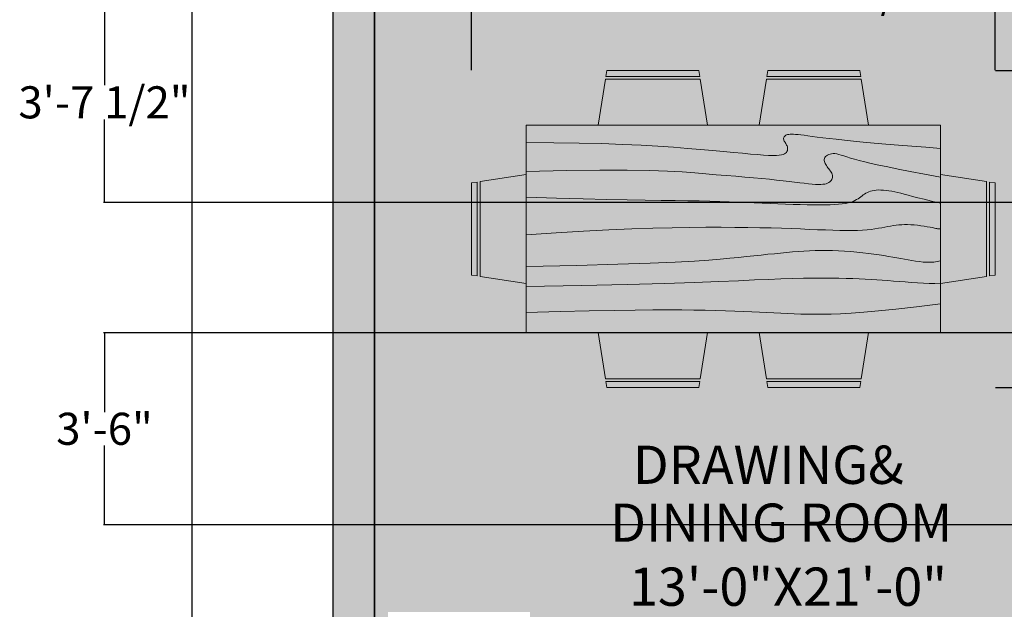
# Model space of a CAD drawing. Units: inches. Extents: x 1884 to 2398, y 474 to 1488.
# Tile 31 of 39: x 1884 to 2099, y 761 to 889. Entities that reach past the tile are written whole.
import ezdxf

# ---------------------------------------------------------------- set-up
doc = ezdxf.new("R2010")
doc.units = ezdxf.units.IN
doc.header["$MEASUREMENT"] = 0
doc.layers.get('0').update_dxf_attribs({"color": 250})
for name, color, linetype, lineweight in [('A-ANNO-DIMS', 2, 'Continuous', 18), ('A-AREA-IDEN', 7, 'Continuous', 18), ('A-FLOR-PATT', 254, 'Continuous', 13), ('A-FURN-PATT', 253, 'Continuous', 13), ('A-WALL-PATT', 250, 'Continuous', 13), ('C-PROP', 7, 'Continuous', 30), ('furniture', 8, 'Continuous', 18), ('walls', 7, 'Continuous', 35)]:
    doc.layers.add(name, color=color, linetype=linetype, lineweight=lineweight)
doc.styles.get("Standard").update_dxf_attribs({"font": 'arial.ttf'})
doc.dimstyles.get("Standard").update_dxf_attribs({"dimtxt": 7, "dimasz": 0.18, "dimexe": 0.18, "dimexo": 0.0625, "dimgap": 0.09, "dimtad": 0, "dimtih": 1, "dimtoh": 1, "dimzin": 0, "dimdsep": 46, "dimlunit": 3, "dimtxsty": 'Standard', "dimcen": 0.09, "dimadec": 0, "dimazin": 0, "dimtfac": 1, "dimtofl": 0, "dimtmove": 0, "dimatfit": 3, "dimfxl": 1, "dimtolj": 1, "dimtzin": 0, "dimarcsym": 0})

# ---------------------------------------------------------------- blocks, each defined once
blk = doc.blocks.new('*D2')
at = {"layer": 'A-ANNO-DIMS', "color": 0, "lineweight": -2, "transparency": 16777216}
for p, q in [((1920.51, 1406.88), (1921.96, 1406.88)), ((1921.78, 1406.7), (1921.78, 972.55)), ((1921.78, 531.06), (1921.78, 965.22)), ((1920.51, 530.88), (1921.96, 530.88))]:
    blk.add_line(p, q, dxfattribs=at)
at = {"layer": 'A-ANNO-DIMS', "color": 0, "lineweight": 100, "transparency": 16777216}
for points in [[(1921.75, 1406.7), (1921.81, 1406.7), (1921.78, 1406.88)], [(1921.75, 531.06), (1921.81, 531.06), (1921.78, 530.88)]]:
    blk.add_solid(points, dxfattribs=at)
at = {"layer": 'Defpoints', "color": 0, "lineweight": 100, "transparency": 16777216}
for p in [(1920.45, 1406.88), (1920.45, 530.88), (1921.78, 530.88)]:
    blk.add_point(p, dxfattribs=at)
at = {"layer": 'A-ANNO-DIMS', "color": 0, "transparency": 16777216, "insert": (1921.78, 968.88), "char_height": 7, "attachment_point": 5}
blk.add_mtext("\\A1;73'", dxfattribs=at)
blk = doc.blocks.new('Dining Set - 36 x 72 in.')
for p, q in [((-22, 27.5), (-22.1562, 26.50042)), ((-22, 27.5), (-6, 27.5)), ((-5.8437, 26.49966), (-6, 27.5)), ((6, 27.5), (5.8438, 26.50042)), ((6, 27.5), (22, 27.5)), ((22.1563, 26.49966), (22, 27.5)), ((-22.2343, 26.00059), (-23.4847, 17.99762)), ((-22.2304, 26), (-5.7608, 26)), ((-5.8416, 26.5), (-22.1534, 26.5)), ((-4.5152, 17.99762), (-5.7655, 25.99926)), ((5.7657, 26.00059), (4.5153, 17.99762)), ((5.7696, 26), (22.2392, 26)), ((22.1584, 26.5), (5.8466, 26.5)), ((23.4848, 17.99762), (22.2345, 25.99926)), ((36, 18), (-36, 18)), ((-36, 18), (-36, -18)), ((36, -18), (36, 18)), ((-44.0006, 8.23428), (-35.9976, 9.48474)), ((44.0006, 8.23428), (35.9976, 9.48474)), ((-45.5, 8), (-44.5004, 8.15617)), ((-45.5, 8), (-45.5, -8)), ((-44.5, -8.15843), (-44.5, 8.15338)), ((-44, 8.23041), (-44, -8.23915)), ((44, 8.23041), (44, -8.23915)), ((44.5, -8.15843), (44.5, 8.15338)), ((45.5, 8), (44.5005, 8.15617)), ((45.5, 8), (45.5, -8)), ((-44.4997, -8.15631), (-45.5, -8)), ((-35.9976, -9.48476), (-43.9993, -8.2345)), ((35.9976, -9.48476), (43.9993, -8.2345)), ((44.4997, -8.15631), (45.5, -8)), ((-36, -18), (36, -18)), ((-22.2343, -26.0006), (-23.4847, -17.99762)), ((-4.5152, -17.99762), (-5.7655, -25.99928)), ((5.7657, -26.0006), (4.5153, -17.99762)), ((23.4848, -17.99762), (22.2345, -25.99928)), ((-22.2304, -26), (-5.7608, -26)), ((-22, -27.5), (-22.1562, -26.50044)), ((-5.8416, -26.5), (-22.1534, -26.5)), ((-5.8437, -26.49967), (-6, -27.5)), ((5.7696, -26), (22.2392, -26)), ((6, -27.5), (5.8438, -26.50044)), ((22.1584, -26.5), (5.8466, -26.5)), ((22.1563, -26.49967), (22, -27.5)), ((-22, -27.5), (-6, -27.5)), ((6, -27.5), (22, -27.5))]:
    blk.add_line(p, q)
for points in [[(-36, 15), (-31.1772, 14.97754), (-26.8079, 14.91406), (-22.8538, 14.81543), (-19.276, 14.6875), (-16.0362, 14.53613), (-13.0957, 14.36718), (-10.4159, 14.18652), (-7.9583, 14), (-5.6904, 13.81315), (-3.6035, 13.63021), (-1.6954, 13.45508), (0.0365, 13.29166), (1.5945, 13.14388), (2.9811, 13.01562), (4.1988, 12.9108), (5.25, 12.83333), (6.1393, 12.78613), (6.8802, 12.76823), (7.4883, 12.77767), (7.9792, 12.8125), (8.3685, 12.87077), (8.6719, 12.95052), (8.9049, 13.0498), (9.0833, 13.16666), (9.2205, 13.29899), (9.3216, 13.44401), (9.3895, 13.59879), (9.4271, 13.76041), (9.4373, 13.92594), (9.4232, 14.09245), (9.3875, 14.257), (9.3333, 14.41666), (9.2638, 14.56917), (9.1836, 14.71484), (9.0975, 14.85465), (9.0104, 14.98958), (8.9272, 15.1206), (8.8529, 15.2487), (8.7922, 15.37483), (8.75, 15.5), (8.7305, 15.62467), (8.7344, 15.74739), (8.7617, 15.86621), (8.8125, 15.97916), (8.8867, 16.08431), (8.9844, 16.17968), (9.1055, 16.26334), (9.25, 16.33333), (9.4189, 16.38802), (9.6172, 16.42708), (9.8506, 16.45052), (10.125, 16.45833), (10.4463, 16.45052), (10.8203, 16.42708), (11.2529, 16.38802), (11.75, 16.33333), (12.3184, 16.26318), (12.9694, 16.17838), (13.7151, 16.07991), (14.5677, 15.96875), (15.5395, 15.84586), (16.6426, 15.71224), (17.8893, 15.56884), (19.2917, 15.41666), (20.859, 15.25667), (22.5879, 15.08984), (24.4721, 14.91715), (26.5052, 14.73958), (28.6809, 14.5581), (30.9929, 14.3737), (33.4347, 14.18733), (36, 14)], [(-36, 10), (-28.9766, 10.14274), (-23.1725, 10.20442), (-18.4241, 10.19775), (-14.5677, 10.13541), (-11.4399, 10.03011), (-8.877, 9.89453), (-6.7154, 9.74137), (-4.7917, 9.58333), (-2.9698, 9.43082), (-1.2246, 9.28515), (0.4415, 9.14534), (2.026, 9.01041), (3.5266, 8.87939), (4.9408, 8.7513), (6.266, 8.62516), (7.5, 8.5), (8.6411, 8.37549), (9.6914, 8.2539), (10.6538, 8.13818), (11.5312, 8.03125), (12.3267, 7.93603), (13.043, 7.85547), (13.6831, 7.79248), (14.25, 7.75), (14.7471, 7.7303), (15.1797, 7.73307), (15.5537, 7.75732), (15.875, 7.80208), (16.1494, 7.86637), (16.3828, 7.94922), (16.5811, 8.04964), (16.75, 8.16666), (16.8944, 8.29915), (17.0143, 8.44531), (17.1089, 8.60319), (17.1771, 8.77083), (17.218, 8.94629), (17.2305, 9.1276), (17.2137, 9.31282), (17.1667, 9.5), (17.0895, 9.6875), (16.987, 9.875), (16.8649, 10.0625), (16.7292, 10.25), (16.5856, 10.4375), (16.4401, 10.625), (16.2985, 10.8125), (16.1667, 11), (16.05, 11.18733), (15.9518, 11.3737), (15.8752, 11.5581), (15.8229, 11.73958), (15.798, 11.91715), (15.8034, 12.08984), (15.842, 12.25667), (15.9167, 12.41666), (16.0295, 12.56836), (16.1784, 12.70833), (16.3605, 12.83268), (16.5729, 12.9375), (16.8127, 13.01888), (17.0768, 13.07291), (17.3625, 13.0957), (17.6667, 13.08333), (17.9894, 13.03312), (18.3418, 12.94726), (18.7382, 12.82918), (19.1927, 12.68229), (19.7195, 12.51001), (20.3327, 12.31575), (21.0465, 12.10294), (21.875, 11.875), (22.8357, 11.63354), (23.959, 11.37304), (25.2786, 11.08618), (26.8282, 10.76562), (28.6414, 10.40405), (30.752, 9.99414), (33.1936, 9.52856), (36, 9)], [(-36, 5.5), (-30.7157, 5.3348), (-26.069, 5.20963), (-21.9946, 5.11767), (-18.4271, 5.05208), (-15.3009, 5.00602), (-12.5508, 4.97265), (-10.1112, 4.94515), (-7.9167, 4.91666), (-5.909, 4.88167), (-4.0586, 4.83984), (-2.3429, 4.79215), (-0.7396, 4.73958), (0.7739, 4.6831), (2.22, 4.6237), (3.6213, 4.56233), (5, 4.5), (6.373, 4.43782), (7.7344, 4.3776), (9.0723, 4.32129), (10.375, 4.27083), (11.6309, 4.22819), (12.8281, 4.19531), (13.9551, 4.17415), (15, 4.16666), (15.954, 4.17448), (16.819, 4.19791), (17.6001, 4.23698), (18.3021, 4.29166), (18.9299, 4.36198), (19.4883, 4.44791), (19.9823, 4.54948), (20.4167, 4.66666), (20.7969, 4.79899), (21.1302, 4.94401), (21.4245, 5.09879), (21.6875, 5.26041), (21.9271, 5.42594), (22.1511, 5.59245), (22.3672, 5.757), (22.5834, 5.91666), (22.8065, 6.06868), (23.0404, 6.21093), (23.2879, 6.34147), (23.5521, 6.45833), (23.8358, 6.55957), (24.142, 6.64323), (24.4735, 6.70735), (24.8334, 6.75), (25.2235, 6.76969), (25.642, 6.76692), (26.0858, 6.74267), (26.5521, 6.69791), (27.0379, 6.63362), (27.5404, 6.55078), (28.0565, 6.45036), (28.5834, 6.33333), (29.1242, 6.19987), (29.7071, 6.04687), (30.3661, 5.87044), (31.1354, 5.66666), (32.0493, 5.43164), (33.142, 5.16146), (34.4475, 4.85221), (36, 4.5)], [(-36, -1), (-30.7915, -0.6591), (-26.0195, -0.38216), (-21.6519, -0.16284), (-17.6563, 0.00521), (-14.0005, 0.12833), (-10.6523, 0.21289), (-7.5796, 0.26522), (-4.75, 0.29166), (-2.134, 0.29793), (0.2878, 0.28711), (2.5317, 0.26163), (4.6146, 0.22396), (6.5529, 0.17651), (8.3633, 0.12174), (10.0623, 0.06209), (11.6667, 0), (13.1899, -0.06201), (14.6341, -0.1211), (15.9982, -0.17432), (17.2813, -0.21875), (18.4823, -0.25147), (19.6003, -0.26953), (20.6343, -0.27002), (21.5834, -0.25), (22.4481, -0.20768), (23.2357, -0.14584), (23.9549, -0.06836), (24.6146, 0.02083), (25.2235, 0.11784), (25.7904, 0.21875), (26.3241, 0.31966), (26.8334, 0.41666), (27.3265, 0.50618), (27.8099, 0.58593), (28.2894, 0.65397), (28.7709, 0.70833), (29.2601, 0.74707), (29.763, 0.76823), (30.2855, 0.76985), (30.8334, 0.75), (31.4088, 0.70784), (31.9994, 0.64713), (32.589, 0.57275), (33.1615, 0.48958), (33.7008, 0.4025), (34.1908, 0.3164), (34.6153, 0.23616), (34.9584, 0.16666), (35.2099, 0.11165), (35.3848, 0.07031), (35.504, 0.04069), (35.5886, 0.02083), (35.6594, 0.00879), (35.7377, 0.0026), (35.8442, 0.00032), (36, 0)], [(-36, -6.5), (-27.1843, -6.31267), (-20.084, -6.1263), (-14.469, -5.9419), (-10.1094, -5.76042), (-6.7752, -5.58285), (-4.2363, -5.41016), (-2.2629, -5.24333), (-0.625, -5.08334), (0.8708, -4.93099), (2.2715, -4.78646), (3.5872, -4.64974), (4.8281, -4.52084), (6.0046, -4.39974), (7.127, -4.28646), (8.2053, -4.18099), (9.25, -4.08334), (10.2705, -3.99382), (11.2734, -3.91407), (12.2647, -3.84603), (13.25, -3.79167), (14.2354, -3.75293), (15.2266, -3.73177), (16.2295, -3.73015), (17.25, -3.75), (18.2912, -3.79248), (19.3451, -3.85547), (20.4009, -3.93604), (21.4479, -4.03125), (22.4754, -4.13819), (23.4727, -4.25391), (24.4289, -4.37549), (25.3334, -4.5), (26.1785, -4.62492), (26.9694, -4.74935), (27.7145, -4.87281), (28.4219, -4.99479), (29.1, -5.11483), (29.7572, -5.23242), (30.4016, -5.34709), (31.0417, -5.45834), (31.6837, -5.56437), (32.3262, -5.65821), (32.9658, -5.73153), (33.599, -5.77604), (34.2224, -5.78345), (34.8327, -5.74545), (35.4264, -5.65373), (36, -5.5)], [(-36, -10), (-26.4022, -9.81299), (-18.4675, -9.62891), (-11.9839, -9.45069), (-6.7396, -9.28125), (-2.5226, -9.12354), (0.8789, -8.98047), (3.6769, -8.85498), (6.0833, -8.75), (8.2767, -8.66765), (10.3021, -8.60677), (12.1712, -8.56543), (13.8958, -8.54167), (15.4876, -8.53353), (16.9583, -8.53907), (18.3197, -8.55632), (19.5834, -8.58334), (20.7616, -8.61841), (21.8685, -8.66081), (22.9188, -8.71004), (23.9271, -8.76563), (24.9081, -8.82707), (25.8763, -8.89388), (26.8465, -8.96558), (27.8334, -9.04167), (28.8474, -9.12118), (29.8828, -9.20117), (30.93, -9.27824), (31.9792, -9.34896), (33.0205, -9.40991), (34.0443, -9.45768), (35.0407, -9.48885), (36, -9.5)], [(-36, -14.5), (-30.0881, -14.33513), (-25.0332, -14.21224), (-20.7312, -14.12647), (-17.0781, -14.07292), (-13.97, -14.04671), (-11.3027, -14.04297), (-8.9724, -14.05681), (-6.875, -14.08334), (-4.9224, -14.11833), (-3.0905, -14.16016), (-1.3709, -14.20785), (0.2448, -14.26042), (1.7647, -14.3169), (3.1973, -14.3763), (4.5507, -14.43767), (5.8333, -14.5), (7.0554, -14.5621), (8.235, -14.62175), (9.3922, -14.67652), (10.5469, -14.72396), (11.7192, -14.76164), (12.929, -14.78711), (14.1965, -14.79794), (15.5417, -14.79167), (16.9933, -14.76424), (18.6152, -14.70508), (20.4804, -14.60197), (22.6615, -14.44271), (25.2312, -14.21509), (28.2624, -13.9069), (31.8277, -13.50594), (36, -13)]]:
    blk.add_lwpolyline(points)
blk = doc.blocks.new('dining area')
at = {"layer": 'furniture', "xscale": 0.6659924291999282, "yscale": 0.6659924291999282, "zscale": 0.6659924291999282, "rotation": 90}
blk.add_blockref('Dining Set - 36 x 72 in.', (-0.44, 20.51), dxfattribs=at)
blk = doc.blocks.new('*D35')
at = {"layer": 'A-ANNO-DIMS', "color": 0, "lineweight": -2, "transparency": 16777216}
for p, q in [((1982.72, 878.09), (1982.72, 895.35)), ((1982.9, 895.17), (1993.17, 895.17)), ((2096.86, 895.17), (2086.6, 895.17)), ((2097.04, 878.09), (2097.04, 895.35))]:
    blk.add_line(p, q, dxfattribs=at)
at = {"layer": 'A-ANNO-DIMS', "color": 0, "lineweight": 100, "transparency": 16777216}
for points in [[(1982.9, 895.2), (1982.9, 895.14), (1982.72, 895.17)], [(2096.86, 895.2), (2096.86, 895.14), (2097.04, 895.17)]]:
    blk.add_solid(points, dxfattribs=at)
at = {"layer": 'Defpoints', "color": 0, "lineweight": 100, "transparency": 16777216}
for p in [(2097.04, 895.17), (1982.72, 878.02), (2097.04, 878.02)]:
    blk.add_point(p, dxfattribs=at)
at = {"layer": 'A-ANNO-DIMS', "color": 0, "transparency": 16777216, "insert": (2039.88, 895.17), "char_height": 7, "attachment_point": 5}
blk.add_mtext('\\A1;DINING SET 9\'-6 1/2"', dxfattribs=at)
blk = doc.blocks.new('*D36')
at = {"layer": 'A-ANNO-DIMS', "color": 0, "lineweight": -2, "transparency": 16777216}
for p, q in [((2097.11, 878.02), (2114.37, 878.02)), ((2114.19, 877.84), (2114.19, 847.14)), ((2114.19, 809.11), (2114.19, 839.81)), ((2097.11, 808.93), (2114.37, 808.93))]:
    blk.add_line(p, q, dxfattribs=at)
at = {"layer": 'A-ANNO-DIMS', "color": 0, "lineweight": 100, "transparency": 16777216}
for points in [[(2114.16, 877.84), (2114.22, 877.84), (2114.19, 878.02)], [(2114.16, 809.11), (2114.22, 809.11), (2114.19, 808.93)]]:
    blk.add_solid(points, dxfattribs=at)
at = {"layer": 'Defpoints', "color": 0, "lineweight": 100, "transparency": 16777216}
for p in [(2097.04, 878.02), (2097.04, 808.93), (2114.19, 808.93)]:
    blk.add_point(p, dxfattribs=at)
at = {"layer": 'A-ANNO-DIMS', "color": 0, "transparency": 16777216, "insert": (2114.19, 843.48), "char_height": 7, "attachment_point": 5}
blk.add_mtext('\\A1;5\'-9"', dxfattribs=at)
blk = doc.blocks.new('*D51')
at = {"layer": 'A-ANNO-DIMS', "color": 0, "lineweight": -2, "transparency": 16777216}
for p, q in [((2202.97, 892.97), (1902.43, 892.97)), ((1902.61, 892.79), (1902.61, 874.82)), ((1902.61, 849.42), (1902.61, 867.39)), ((2202.97, 849.24), (1902.43, 849.24))]:
    blk.add_line(p, q, dxfattribs=at)
at = {"layer": 'A-ANNO-DIMS', "color": 0, "lineweight": 100, "transparency": 16777216}
for points in [[(1902.58, 892.79), (1902.64, 892.79), (1902.61, 892.97)], [(1902.58, 849.42), (1902.64, 849.42), (1902.61, 849.24)]]:
    blk.add_solid(points, dxfattribs=at)
at = {"layer": 'Defpoints', "color": 0, "lineweight": 100, "transparency": 16777216}
for p in [(1902.61, 892.97), (2203.03, 892.97), (2203.03, 849.24)]:
    blk.add_point(p, dxfattribs=at)
at = {"layer": 'A-ANNO-DIMS', "color": 0, "transparency": 16777216, "insert": (1902.61, 871.1), "char_height": 7, "attachment_point": 5}
blk.add_mtext('\\A1;3\'-7 1/2"', dxfattribs=at)
blk = doc.blocks.new('*D53')
at = {"layer": 'A-ANNO-DIMS', "color": 0, "lineweight": -2, "transparency": 16777216}
for p, q in [((2262.32, 820.83), (1902.43, 820.83)), ((1902.61, 820.65), (1902.61, 803.56)), ((1902.61, 779.15), (1902.61, 796.23)), ((2262.32, 778.97), (1902.43, 778.97))]:
    blk.add_line(p, q, dxfattribs=at)
at = {"layer": 'A-ANNO-DIMS', "color": 0, "lineweight": 100, "transparency": 16777216}
for points in [[(1902.58, 820.65), (1902.64, 820.65), (1902.61, 820.83)], [(1902.58, 779.15), (1902.64, 779.15), (1902.61, 778.97)]]:
    blk.add_solid(points, dxfattribs=at)
at = {"layer": 'Defpoints', "color": 0, "lineweight": 100, "transparency": 16777216}
for p in [(1902.61, 820.83), (2262.38, 820.83), (2262.38, 778.97)]:
    blk.add_point(p, dxfattribs=at)
at = {"layer": 'A-ANNO-DIMS', "color": 0, "transparency": 16777216, "insert": (1902.61, 799.9), "char_height": 7, "attachment_point": 5}
blk.add_mtext('\\A1;3\'-6"', dxfattribs=at)

msp = doc.modelspace()

# ---------------------------------------------------------------- hatches: boundary and pattern name
at = {"layer": 'A-FLOR-PATT'}
h = msp.add_hatch(color=256, dxfattribs=at)
h.dxf.hatch_style = 1
h.paths.add_polyline_path([(2117.529, 815.801), (2126.529, 815.801), (2126.529, 880.382), (2117.529, 880.382), (2117.529, 892.385), (1961.529, 892.385), (1961.529, 756.915), (1964.529, 756.915), (1964.529, 759.915), (1995.529, 759.915), (1995.529, 753.915), (1972.862, 753.915), (1967.529, 756.915), (1967.529, 654.915), (1972.862, 657.915), (1995.529, 657.915), (1995.529, 651.915), (1964.529, 651.915), (1964.529, 654.915), (1961.529, 654.915), (1961.529, 640.385), (2117.529, 640.385), (2117.529, 646.578), (2126.529, 646.578), (2126.529, 676.183), (2117.529, 676.183)])
h.paths.add_polyline_path([(2012.246, 808.929), (2012.05, 810.185), (2032.542, 810.185), (2032.346, 808.929)], flags=16)
h.paths.add_polyline_path([(2010.381, 820.864), (1994.658, 820.864), (1994.658, 831.561), (1984.608, 833.132), (1984.608, 853.821), (1994.658, 855.391), (1994.658, 866.089), (2010.381, 866.089), (2011.951, 876.139), (2032.64, 876.139), (2034.211, 866.089), (2045.556, 866.089), (2047.127, 876.139), (2067.816, 876.139), (2069.386, 866.089), (2085.109, 866.089), (2085.109, 855.391), (2095.159, 853.821), (2095.159, 833.132), (2085.109, 831.561), (2085.109, 820.864), (2069.386, 820.864), (2067.816, 810.814), (2047.127, 810.814), (2045.556, 820.864), (2034.211, 820.864), (2032.64, 810.814), (2011.951, 810.814)], flags=16)
h.paths.add_polyline_path([(1982.724, 833.426), (1982.724, 853.526), (1983.98, 853.723), (1983.98, 833.23)], flags=16)
h.paths.add_polyline_path([(1994.529, 753.54), (1994.529, 658.29), (1973.529, 658.29), (1973.529, 753.54)], flags=16)
h.paths.add_polyline_path([(2084.486, 843.527), (2084.592, 843.502), (2084.681, 843.487), (2084.813, 843.477), (2084.913, 843.477), (2084.669, 843.482), (2084.336, 843.565), (2084.116, 843.617), (2083.8, 843.686), (2083.105, 843.827), (2082.836, 843.874), (2083.604, 843.729), (2084.206, 843.597)], flags=0)
h.paths.add_polyline_path([(2047.421, 808.929), (2047.225, 810.185), (2067.718, 810.185), (2067.521, 808.929)], flags=16)
h.paths.add_polyline_path([(2066.01, 849.505), (2066.429, 849.687), (2066.798, 849.882), (2067.129, 850.085), (2067.43, 850.293), (2067.711, 850.502), (2068.176, 850.856), (2068.689, 851.205), (2069.305, 851.531), (2070.015, 851.784), (2070.844, 851.944), (2071.081, 851.956), (2070.629, 851.902), (2070.212, 851.822), (2069.827, 851.717), (2069.471, 851.59), (2069.139, 851.443), (2068.828, 851.279), (2068.534, 851.1), (2068.254, 850.909), (2067.983, 850.709), (2067.502, 850.343), (2066.951, 849.962), (2066.224, 849.579)], flags=0)
h.paths.add_polyline_path([(2059.423, 853.221), (2059.827, 853.278), (2060.171, 853.358), (2060.465, 853.463), (2060.714, 853.589), (2060.926, 853.736), (2061.107, 853.902), (2061.258, 854.086), (2061.377, 854.284), (2061.462, 854.495), (2061.514, 854.715), (2061.53, 854.943), (2061.508, 855.176), (2061.449, 855.411), (2061.352, 855.646), (2061.224, 855.882), (2061.07, 856.117), (2060.9, 856.353), (2060.719, 856.588), (2060.406, 856.993), (2060.103, 857.424), (2059.858, 857.888), (2059.691, 858.467), (2059.836, 859.091), (2060.305, 859.532), (2060.844, 859.798), (2061.513, 859.935), (2062.253, 859.905), (2062.483, 859.849), (2062.078, 859.912), (2061.695, 859.928), (2061.336, 859.899), (2061.005, 859.831), (2060.703, 859.729), (2060.437, 859.597), (2060.208, 859.441), (2060.021, 859.265), (2059.879, 859.075), (2059.785, 858.874), (2059.737, 858.664), (2059.73, 858.447), (2059.761, 858.224), (2059.827, 857.996), (2059.923, 857.765), (2060.047, 857.53), (2060.193, 857.295), (2060.359, 857.06), (2060.537, 856.824), (2060.867, 856.399), (2061.171, 855.978), (2061.422, 855.518), (2061.567, 854.943), (2061.41, 854.272), (2060.947, 853.707), (2060.335, 853.397), (2059.649, 853.236)], flags=0)
h.paths.add_polyline_path([(2050.778, 859.745), (2051.07, 859.87), (2051.295, 860.017), (2051.467, 860.183), (2051.594, 860.365), (2051.679, 860.56), (2051.726, 860.763), (2051.739, 860.971), (2051.722, 861.18), (2051.677, 861.387), (2051.609, 861.587), (2051.521, 861.779), (2051.421, 861.962), (2051.312, 862.138), (2051.203, 862.307), (2050.966, 862.68), (2050.793, 863.193), (2051.021, 863.699), (2051.483, 864.018), (2052.09, 864.138), (2052.773, 864.157), (2053.007, 864.142), (2052.603, 864.152), (2052.258, 864.142), (2051.965, 864.113), (2051.716, 864.064), (2051.504, 863.995), (2051.322, 863.907), (2051.17, 863.802), (2051.048, 863.682), (2050.954, 863.55), (2050.891, 863.408), (2050.856, 863.259), (2050.851, 863.105), (2050.876, 862.948), (2050.929, 862.791), (2051.005, 862.633), (2051.098, 862.472), (2051.203, 862.307), (2051.312, 862.138), (2051.556, 861.742), (2051.751, 861.167), (2051.712, 860.535), (2051.398, 860.085), (2050.949, 859.79)], flags=0)
h.paths.add_polyline_path([(2022.768, 719.264), (2050.461, 719.264), (2050.461, 717.226), (2052.426, 717.226), (2052.426, 715.033), (2050.461, 715.033), (2050.461, 703.738), (2022.768, 703.738)], flags=16)
h.paths.add_polyline_path([(2012.246, 878.023), (2032.346, 878.023), (2032.542, 876.767), (2012.05, 876.767)], flags=16)
h.paths.add_polyline_path([(2035.324, 713.103), (2035.342, 713.294), (2035.192, 713.202)], flags=0)
h.paths.add_polyline_path([(2036.484, 711.63), (2036.583, 711.849), (2036.39, 711.898)], flags=0)
h.paths.add_polyline_path([(2036.074, 712.744), (2035.993, 712.481), (2035.724, 712.516), (2035.794, 712.726)], flags=0)
h.paths.add_polyline_path([(2035.846, 710.909), (2035.753, 710.958), (2035.702, 710.88)], flags=0)
h.paths.add_polyline_path([(2037.818, 712.019), (2037.948, 712.06), (2037.987, 712.161), (2037.815, 712.02)], flags=0)
h.paths.add_polyline_path([(2038.451, 709.517), (2038.464, 709.428), (2038.586, 709.442)], flags=0)
h.paths.add_polyline_path([(2037.805, 709.806), (2037.818, 709.807), (2037.804, 709.823)], flags=0)
h.paths.add_polyline_path([(2036.7, 711.245), (2036.698, 711.236), (2036.813, 711.211)], flags=0)
h.paths.add_polyline_path([(2035.928, 708.897), (2035.668, 708.871), (2035.706, 708.667)], flags=0)
h.paths.add_polyline_path([(2036.414, 710.976), (2035.932, 709.859), (2036.792, 710.484), (2036.5, 710.934)], flags=0)
h.paths.add_polyline_path([(2038.298, 712.115), (2038.499, 712.058), (2038.612, 712.269), (2038.39, 712.332)], flags=0)
h.paths.add_polyline_path([(2047.421, 878.023), (2067.521, 878.023), (2067.718, 876.767), (2047.225, 876.767)], flags=16)
h.paths.add_polyline_path([(2049.647, 705.093, -1), (2048.845, 705.093, -1)], flags=0)
h.paths.add_polyline_path([(2095.787, 853.723), (2097.043, 853.526), (2097.043, 833.426), (2095.787, 833.23)], flags=16)
h.paths.add_polyline_path([(2110.739, 745.339), (2111.75, 745.339, -0.0640419), (2113.267, 742.92), (2113.267, 732.192), (2113.526, 732.192, -0.4142136), (2114.278, 731.439), (2114.278, 716.764, -0.4142136), (2113.526, 716.011), (2113.267, 716.011), (2113.267, 705.284, -0.0640419), (2111.75, 702.864), (2110.739, 702.864), (2110.739, 716.011), (2109.469, 716.011, -0.4142136), (2108.716, 716.764), (2108.716, 731.439, -0.4142136), (2109.469, 732.192), (2110.739, 732.192)], flags=16)
h.paths.add_polyline_path([(1998.045, 668.909), (2002.449, 668.909), (2002.449, 652.273), (2002.724, 652.763), (2002.724, 668.175), (2019.972, 668.175), (2019.972, 652.763), (2020.247, 652.273), (2020.247, 668.909), (2024.651, 668.909), (2029.055, 668.909), (2029.055, 652.273), (2029.33, 652.763), (2029.33, 668.175), (2046.578, 668.175), (2046.578, 652.763), (2046.853, 652.273), (2046.853, 668.909), (2051.257, 668.909), (2051.257, 646.157), (2049.055, 646.157), (2049.055, 643.955), (2026.853, 643.955), (2026.853, 646.157), (2024.651, 646.157), (2022.449, 646.157), (2022.449, 643.955), (2000.247, 643.955), (2000.247, 646.157), (1998.045, 646.157)], flags=16)
h.paths.add_polyline_path([(2342.529, 1247.885), (2265.892, 1247.885), (2230.029, 1247.885), (2209.755, 1247.885), (2168.6, 1247.885), (2168.6, 1104.929), (2158.029, 1104.929), (2158.029, 1079.411), (2168.6, 1079.411), (2168.6, 1062.466), (2342.529, 1062.466), (2342.529, 1093.809)])
h.paths.add_polyline_path([(2215.03, 1153.876), (2215.03, 1164.739), (2187.559, 1164.739), (2187.442, 1152.641), (2173.568, 1152.641), (2173.684, 1164.739), (2173.684, 1218.739), (2173.801, 1230.837), (2187.675, 1230.837), (2187.559, 1218.739), (2215.03, 1218.739), (2215.03, 1225.879), (2245.053, 1225.879), (2245.053, 1153.876)], flags=16)
h.paths.add_polyline_path([(2192.147, 1164.797), (2184.963, 1174.54), (2184.915, 1174.54), (2176.755, 1174.54), (2176.755, 1190.363), (2184.915, 1190.363), (2184.915, 1196.819), (2176.755, 1196.819), (2176.755, 1212.641), (2184.915, 1212.641), (2184.915, 1174.606), (2184.963, 1174.54), (2192.147, 1174.54)], flags=0)
h.paths.add_polyline_path([(2184.971, 1158.364, -1), (2176.039, 1158.364, -1)], flags=0)
h.paths.add_polyline_path([(2335.555, 1161.985), (2335.555, 1175.132), (2334.285, 1175.132, -0.4142136), (2333.533, 1175.885), (2333.533, 1190.56, -0.4142136), (2334.285, 1191.313), (2335.555, 1191.313), (2335.555, 1204.46), (2336.567, 1204.46, -0.0640419), (2338.083, 1202.04), (2338.083, 1191.313), (2338.342, 1191.313, -0.4142136), (2339.095, 1190.56), (2339.095, 1175.885, -0.4142136), (2338.342, 1175.132), (2338.083, 1175.132), (2338.083, 1164.405, -0.0640419), (2336.567, 1161.985)], flags=16)
h.paths.add_polyline_path([(2176.155, 1224.462, -1), (2185.087, 1224.462, -1)], flags=0)
h.paths.add_polyline_path([(2158.029, 1276.197), (2158.029, 1322.885), (2148.233, 1322.885), (2092.029, 1322.885), (1961.529, 1322.885), (1961.529, 1166.885), (2116.005, 1166.885), (2116.005, 1157.885), (2152.638, 1157.885), (2152.638, 1166.885), (2158.029, 1166.885)])
h.paths.add_polyline_path([(2006.352, 1204.245), (2006.352, 1215.108), (1978.881, 1215.108), (1978.764, 1203.01), (1964.89, 1203.01), (1965.006, 1215.108), (1965.006, 1269.108), (1965.123, 1281.207), (1978.997, 1281.207), (1978.881, 1269.108), (2006.352, 1269.108), (2006.352, 1276.248), (2036.375, 1276.248), (2036.375, 1204.245)], flags=16)
h.paths.add_polyline_path([(1983.469, 1215.166), (1976.285, 1224.909), (1976.237, 1224.909), (1968.077, 1224.909), (1968.077, 1240.732), (1976.237, 1240.732), (1976.237, 1247.188), (1968.077, 1247.188), (1968.077, 1263.011), (1976.237, 1263.011), (1976.237, 1224.975), (1976.285, 1224.909), (1983.469, 1224.909)], flags=0)
h.paths.add_polyline_path([(1976.293, 1208.733, -1), (1967.361, 1208.733, -1)], flags=0)
h.paths.add_polyline_path([(1967.477, 1274.832, -1), (1976.41, 1274.832, -1)], flags=0)
h.paths.add_polyline_path([(2152.587, 1223.485), (2152.587, 1236.632), (2151.317, 1236.632, -0.4142136), (2150.564, 1237.385), (2150.564, 1252.06, -0.4142136), (2151.317, 1252.813), (2152.587, 1252.813), (2152.587, 1265.959), (2153.598, 1265.959, -0.0640419), (2155.115, 1263.54), (2155.115, 1252.813), (2155.374, 1252.813, -0.4142136), (2156.126, 1252.06), (2156.126, 1237.385, -0.4142136), (2155.374, 1236.632), (2155.115, 1236.632), (2155.115, 1225.904, -0.0640419), (2153.598, 1223.485)], flags=16)
h.paths.add_polyline_path([(2250.676, 1161.101), (2322.077, 1161.101), (2322.077, 1173.886), (2250.676, 1173.886)], flags=24)
h.paths.add_polyline_path([(2255.61, 1173.712), (2320.136, 1173.712), (2320.136, 1186.659), (2255.61, 1186.659)], flags=24)
h.paths.add_polyline_path([(2053.687, 1230.837), (2125.089, 1230.837), (2125.089, 1243.622), (2053.687, 1243.622)], flags=24)
h.paths.add_polyline_path([(2058.622, 1243.448), (2123.147, 1243.448), (2123.147, 1256.395), (2058.622, 1256.395)], flags=24)
at = {"layer": 'A-FURN-PATT'}
h = msp.add_hatch(color=256, dxfattribs=at)
h.dxf.hatch_style = 1
h.paths.add_polyline_path([(2032.64, 876.139), (2011.951, 876.139), (2010.381, 866.089), (2034.211, 866.089)])
h.paths.add_polyline_path([(2032.346, 878.023), (2012.246, 878.023), (2012.05, 876.767), (2032.542, 876.767)])
h.paths.add_polyline_path([(2067.816, 876.139), (2047.127, 876.139), (2045.556, 866.089), (2069.386, 866.089)])
h.paths.add_polyline_path([(2067.521, 878.023), (2047.421, 878.023), (2047.225, 876.767), (2067.718, 876.767)])
h.paths.add_polyline_path([(2095.159, 853.821), (2085.109, 855.391), (2085.109, 831.561), (2095.159, 833.132)])
h.paths.add_polyline_path([(2097.043, 853.526), (2095.787, 853.723), (2095.787, 833.23), (2097.043, 833.426)])
h.paths.add_polyline_path([(2069.386, 820.864), (2045.556, 820.864), (2047.127, 810.814), (2067.816, 810.814)])
h.paths.add_polyline_path([(2067.718, 810.185), (2047.225, 810.185), (2047.421, 808.929), (2067.521, 808.929)])
h.paths.add_polyline_path([(2034.211, 820.864), (2010.381, 820.864), (2011.951, 810.814), (2032.64, 810.814)])
h.paths.add_polyline_path([(2032.542, 810.185), (2012.05, 810.185), (2012.246, 808.929), (2032.346, 808.929)])
h.paths.add_polyline_path([(1994.658, 855.391), (1984.608, 853.821), (1984.608, 833.132), (1994.658, 831.561)])
h.paths.add_polyline_path([(1983.98, 853.723), (1982.724, 853.526), (1982.724, 833.426), (1983.98, 833.23)])
h = msp.add_hatch(color=256, dxfattribs=at)
h.dxf.hatch_style = 1
h.paths.add_polyline_path([(2050.987, 863.624), (2051.234, 863.865), (2051.504, 863.995), (2051.716, 864.064), (2051.965, 864.113), (2052.258, 864.142), (2052.603, 864.152), (2053.007, 864.142), (2053.477, 864.113), (2054.02, 864.064), (2054.645, 863.995), (2055.359, 863.907), (2056.176, 863.801), (2057.113, 863.677), (2058.184, 863.537), (2059.405, 863.383), (2060.791, 863.215), (2062.357, 863.035), (2064.119, 862.844), (2066.088, 862.643), (2068.26, 862.433), (2070.627, 862.216), (2073.181, 861.993), (2075.914, 861.765), (2078.819, 861.533), (2081.886, 861.299), (2085.109, 861.064), (2085.109, 866.089), (1994.658, 866.089), (1994.658, 862.32), (2000.717, 862.292), (2006.206, 862.212), (2011.173, 862.088), (2015.668, 861.928), (2019.738, 861.737), (2023.432, 861.525), (2026.799, 861.298), (2029.886, 861.064), (2032.735, 860.829), (2035.357, 860.599), (2037.754, 860.379), (2039.929, 860.174), (2041.887, 859.988), (2043.629, 859.827), (2045.158, 859.696), (2046.479, 859.598), (2047.596, 859.539), (2048.527, 859.516), (2049.291, 859.528), (2049.908, 859.572), (2050.397, 859.645), (2050.778, 859.745), (2051.07, 859.87), (2051.295, 860.017), (2051.467, 860.183), (2051.594, 860.365), (2051.679, 860.56), (2051.726, 860.763), (2051.739, 860.971), (2051.722, 861.18), (2051.677, 861.387), (2051.609, 861.587), (2051.521, 861.779), (2051.421, 861.962), (2051.312, 862.138), (2051.114, 862.445), (2050.951, 862.727), (2050.849, 863.028), (2050.859, 863.338)])
h.paths.add_polyline_path([(2060.021, 859.265), (2060.208, 859.441), (2060.437, 859.597), (2060.703, 859.729), (2061.005, 859.831), (2061.336, 859.899), (2061.695, 859.928), (2062.078, 859.912), (2062.483, 859.849), (2062.926, 859.741), (2063.424, 859.593), (2063.995, 859.409), (2064.656, 859.192), (2065.427, 858.948), (2066.323, 858.681), (2067.364, 858.394), (2068.571, 858.091), (2069.982, 857.764), (2071.64, 857.403), (2073.587, 857.001), (2075.865, 856.546), (2078.516, 856.032), (2081.583, 855.447), (2085.109, 854.783), (2085.109, 861.064), (2081.886, 861.299), (2078.819, 861.533), (2075.914, 861.765), (2073.181, 861.993), (2070.627, 862.216), (2068.26, 862.433), (2066.088, 862.643), (2064.119, 862.844), (2062.357, 863.035), (2060.791, 863.215), (2059.405, 863.383), (2058.184, 863.537), (2057.113, 863.677), (2056.176, 863.801), (2055.359, 863.907), (2054.645, 863.995), (2054.02, 864.064), (2053.477, 864.113), (2053.007, 864.142), (2052.603, 864.152), (2052.258, 864.142), (2051.965, 864.113), (2051.716, 864.064), (2051.504, 863.995), (2051.322, 863.907), (2051.17, 863.802), (2051.048, 863.682), (2050.954, 863.55), (2050.891, 863.408), (2050.856, 863.259), (2050.851, 863.105), (2050.876, 862.948), (2050.929, 862.791), (2051.005, 862.633), (2051.098, 862.472), (2051.203, 862.307), (2051.39, 862.017), (2051.579, 861.673), (2051.713, 861.279), (2051.749, 860.859), (2051.654, 860.452), (2051.467, 860.183), (2051.295, 860.017), (2051.07, 859.87), (2050.778, 859.745), (2050.397, 859.645), (2049.908, 859.572), (2049.291, 859.528), (2048.527, 859.516), (2047.596, 859.539), (2046.479, 859.598), (2045.158, 859.696), (2043.629, 859.827), (2041.887, 859.988), (2039.929, 860.174), (2037.754, 860.379), (2035.357, 860.599), (2032.735, 860.829), (2029.886, 861.064), (2026.799, 861.298), (2023.432, 861.525), (2019.738, 861.737), (2015.668, 861.928), (2011.173, 862.088), (2006.206, 862.212), (2000.717, 862.292), (1994.658, 862.32), (1994.658, 856.039), (2003.481, 856.218), (2010.773, 856.296), (2016.738, 856.287), (2021.583, 856.209), (2025.512, 856.077), (2028.732, 855.906), (2031.447, 855.714), (2033.864, 855.515), (2036.153, 855.324), (2038.345, 855.141), (2040.438, 854.965), (2042.429, 854.796), (2044.314, 854.631), (2046.09, 854.47), (2047.755, 854.312), (2049.306, 854.154), (2050.739, 853.998), (2052.058, 853.845), (2053.267, 853.7), (2054.37, 853.566), (2055.369, 853.446), (2056.269, 853.345), (2057.073, 853.266), (2057.785, 853.212), (2058.41, 853.188), (2058.953, 853.191), (2059.423, 853.221), (2059.827, 853.278), (2060.171, 853.358), (2060.465, 853.463), (2060.714, 853.589), (2060.926, 853.736), (2061.107, 853.902), (2061.258, 854.086), (2061.377, 854.284), (2061.462, 854.495), (2061.514, 854.715), (2061.53, 854.943), (2061.508, 855.176), (2061.449, 855.411), (2061.352, 855.646), (2061.224, 855.882), (2061.07, 856.117), (2060.9, 856.353), (2060.719, 856.588), (2060.406, 856.993), (2060.193, 857.295), (2060.047, 857.53), (2059.923, 857.765), (2059.776, 858.119), (2059.714, 858.564), (2059.785, 858.874), (2059.879, 859.075)])
h.paths.add_polyline_path([(2071.571, 851.981), (2072.097, 851.977), (2072.654, 851.947), (2073.24, 851.891), (2073.85, 851.81), (2074.481, 851.706), (2075.13, 851.58), (2075.792, 851.433), (2076.471, 851.265), (2077.203, 851.073), (2078.031, 850.851), (2078.998, 850.595), (2080.146, 850.3), (2081.518, 849.96), (2083.159, 849.572), (2085.109, 849.129), (2085.109, 854.783), (2081.583, 855.447), (2078.516, 856.032), (2075.865, 856.546), (2073.587, 857.001), (2071.64, 857.403), (2069.982, 857.764), (2068.571, 858.091), (2067.364, 858.394), (2066.323, 858.681), (2065.427, 858.948), (2064.656, 859.192), (2063.995, 859.409), (2063.424, 859.593), (2062.926, 859.741), (2062.483, 859.849), (2062.078, 859.912), (2061.695, 859.928), (2061.336, 859.899), (2061.005, 859.831), (2060.703, 859.729), (2060.437, 859.597), (2060.208, 859.441), (2060.021, 859.265), (2059.879, 859.075), (2059.785, 858.874), (2059.737, 858.664), (2059.73, 858.447), (2059.761, 858.224), (2059.827, 857.996), (2059.923, 857.765), (2060.047, 857.53), (2060.193, 857.295), (2060.359, 857.06), (2060.537, 856.824), (2060.719, 856.588), (2061.014, 856.204), (2061.224, 855.882), (2061.352, 855.646), (2061.449, 855.411), (2061.508, 855.176), (2061.53, 854.943), (2061.514, 854.715), (2061.462, 854.495), (2061.377, 854.284), (2061.258, 854.086), (2061.107, 853.902), (2060.926, 853.736), (2060.714, 853.589), (2060.465, 853.463), (2060.171, 853.358), (2059.827, 853.278), (2059.423, 853.221), (2058.953, 853.191), (2058.41, 853.188), (2057.785, 853.212), (2057.073, 853.266), (2056.269, 853.345), (2055.369, 853.446), (2054.37, 853.566), (2053.267, 853.7), (2052.058, 853.845), (2050.739, 853.998), (2049.306, 854.154), (2047.755, 854.312), (2046.09, 854.47), (2044.314, 854.631), (2042.429, 854.796), (2040.438, 854.965), (2038.345, 855.141), (2036.153, 855.324), (2033.864, 855.515), (2031.447, 855.714), (2028.732, 855.906), (2025.512, 856.077), (2021.583, 856.209), (2016.738, 856.287), (2010.773, 856.296), (2003.481, 856.218), (1994.658, 856.039), (1994.658, 850.386), (2001.297, 850.178), (2007.134, 850.021), (2012.253, 849.905), (2016.734, 849.823), (2020.662, 849.765), (2024.117, 849.723), (2027.181, 849.689), (2029.938, 849.653), (2032.46, 849.609), (2034.785, 849.556), (2036.94, 849.496), (2038.954, 849.43), (2040.856, 849.359), (2042.672, 849.285), (2044.433, 849.208), (2046.165, 849.129), (2047.89, 849.051), (2049.6, 848.976), (2051.281, 848.905), (2052.917, 848.842), (2054.495, 848.788), (2055.999, 848.747), (2057.415, 848.72), (2058.727, 848.711), (2059.926, 848.721), (2061.013, 848.75), (2061.994, 848.799), (2062.876, 848.868), (2063.664, 848.956), (2064.366, 849.064), (2064.987, 849.192), (2065.532, 849.339), (2066.01, 849.505), (2066.429, 849.687), (2066.798, 849.882), (2067.129, 850.085), (2067.43, 850.293), (2067.711, 850.502), (2067.983, 850.709), (2068.254, 850.909), (2068.534, 851.1), (2068.828, 851.279), (2069.139, 851.443), (2069.471, 851.59), (2069.827, 851.717), (2070.212, 851.822), (2070.629, 851.902), (2071.081, 851.956)])
h.paths.add_polyline_path([(2085.109, 849.129), (2083.159, 849.572), (2081.518, 849.96), (2080.146, 850.3), (2078.998, 850.595), (2078.031, 850.851), (2077.203, 851.073), (2076.471, 851.265), (2075.792, 851.433), (2075.13, 851.58), (2074.481, 851.706), (2073.85, 851.81), (2073.24, 851.891), (2072.654, 851.947), (2072.097, 851.977), (2071.571, 851.981), (2071.081, 851.956), (2070.629, 851.902), (2070.212, 851.822), (2069.827, 851.717), (2069.471, 851.59), (2069.139, 851.443), (2068.828, 851.279), (2068.534, 851.1), (2068.254, 850.909), (2067.983, 850.709), (2067.711, 850.502), (2067.43, 850.293), (2067.129, 850.085), (2066.798, 849.882), (2066.429, 849.687), (2066.01, 849.505), (2065.532, 849.339), (2064.987, 849.192), (2064.366, 849.064), (2063.664, 848.956), (2062.876, 848.868), (2061.994, 848.799), (2061.013, 848.75), (2059.926, 848.721), (2058.727, 848.711), (2057.415, 848.72), (2055.999, 848.747), (2054.495, 848.788), (2052.917, 848.842), (2051.281, 848.905), (2049.6, 848.976), (2047.89, 849.051), (2046.165, 849.129), (2044.433, 849.208), (2042.672, 849.285), (2040.856, 849.359), (2038.954, 849.43), (2036.94, 849.496), (2034.785, 849.556), (2032.46, 849.609), (2029.938, 849.653), (2027.181, 849.689), (2024.117, 849.723), (2020.662, 849.765), (2016.734, 849.823), (2012.253, 849.905), (2007.134, 850.021), (2001.297, 850.178), (1994.658, 850.386), (1994.658, 842.22), (2001.201, 842.648), (2007.196, 842.996), (2012.683, 843.272), (2017.703, 843.483), (2022.295, 843.638), (2026.502, 843.744), (2030.362, 843.809), (2033.916, 843.843), (2037.203, 843.851), (2040.245, 843.837), (2043.064, 843.805), (2045.681, 843.758), (2048.116, 843.698), (2050.39, 843.629), (2052.524, 843.554), (2054.54, 843.476), (2056.453, 843.398), (2058.268, 843.324), (2059.981, 843.257), (2061.593, 843.201), (2063.102, 843.16), (2064.507, 843.138), (2065.806, 843.137), (2066.998, 843.162), (2068.084, 843.215), (2069.074, 843.293), (2069.977, 843.39), (2070.806, 843.502), (2071.571, 843.624), (2072.283, 843.751), (2072.953, 843.878), (2073.593, 844), (2074.213, 844.112), (2074.82, 844.212), (2075.422, 844.298), (2076.027, 844.366), (2076.642, 844.415), (2077.274, 844.441), (2077.93, 844.443), (2078.618, 844.418), (2079.341, 844.366), (2080.083, 844.289), (2080.824, 844.196), (2081.543, 844.091), (2082.22, 843.982), (2082.836, 843.874), (2083.369, 843.773), (2083.8, 843.686), (2084.116, 843.617), (2084.336, 843.565), (2084.486, 843.527), (2084.592, 843.502), (2084.681, 843.487), (2084.779, 843.48), (2084.913, 843.477), (2085.109, 843.476)])
h.paths.add_polyline_path([(2085.109, 843.476), (2084.741, 843.477), (2084.573, 843.506), (2084.336, 843.565), (2084.116, 843.617), (2083.8, 843.686), (2083.369, 843.773), (2082.836, 843.874), (2082.22, 843.982), (2081.543, 844.091), (2080.824, 844.196), (2080.083, 844.289), (2079.341, 844.366), (2078.618, 844.418), (2077.93, 844.443), (2077.274, 844.441), (2076.642, 844.415), (2076.027, 844.366), (2075.422, 844.298), (2074.82, 844.212), (2074.213, 844.112), (2073.593, 844), (2072.953, 843.878), (2072.283, 843.751), (2071.571, 843.624), (2070.806, 843.502), (2069.977, 843.39), (2069.074, 843.293), (2068.084, 843.215), (2066.998, 843.162), (2065.806, 843.137), (2064.507, 843.138), (2063.102, 843.16), (2061.593, 843.201), (2059.981, 843.257), (2058.268, 843.324), (2056.453, 843.398), (2054.54, 843.476), (2052.524, 843.554), (2050.39, 843.629), (2048.116, 843.698), (2045.681, 843.758), (2043.064, 843.805), (2040.245, 843.837), (2037.203, 843.851), (2033.916, 843.843), (2030.362, 843.809), (2026.502, 843.744), (2022.295, 843.638), (2017.703, 843.483), (2012.683, 843.272), (2007.196, 842.996), (2001.201, 842.648), (1994.658, 842.22), (1994.658, 835.311), (2005.733, 835.546), (2014.653, 835.78), (2021.707, 836.012), (2027.184, 836.24), (2031.372, 836.463), (2034.562, 836.68), (2037.041, 836.889), (2039.098, 837.09), (2040.978, 837.282), (2042.737, 837.463), (2044.39, 837.635), (2045.949, 837.797), (2047.427, 837.949), (2048.837, 838.091), (2050.192, 838.224), (2051.504, 838.347), (2052.786, 838.459), (2054.046, 838.559), (2055.291, 838.645), (2056.529, 838.713), (2057.767, 838.762), (2059.012, 838.788), (2060.272, 838.79), (2061.554, 838.765), (2062.862, 838.712), (2064.186, 838.633), (2065.512, 838.532), (2066.828, 838.412), (2068.118, 838.278), (2069.371, 838.132), (2070.573, 837.98), (2071.709, 837.823), (2072.771, 837.666), (2073.764, 837.51), (2074.7, 837.355), (2075.589, 837.202), (2076.441, 837.051), (2077.266, 836.903), (2078.076, 836.759), (2078.88, 836.619), (2079.686, 836.486), (2080.494, 836.368), (2081.297, 836.276), (2082.093, 836.22), (2082.876, 836.211), (2083.642, 836.259), (2084.388, 836.374), (2085.109, 836.567)])
h.paths.add_polyline_path([(2085.109, 836.567), (2084.388, 836.374), (2083.642, 836.259), (2082.876, 836.211), (2082.093, 836.22), (2081.297, 836.276), (2080.494, 836.368), (2079.686, 836.486), (2078.88, 836.619), (2078.076, 836.759), (2077.266, 836.903), (2076.441, 837.051), (2075.589, 837.202), (2074.7, 837.355), (2073.764, 837.51), (2072.771, 837.666), (2071.709, 837.823), (2070.573, 837.98), (2069.371, 838.132), (2068.118, 838.278), (2066.828, 838.412), (2065.512, 838.532), (2064.186, 838.633), (2062.862, 838.712), (2061.554, 838.765), (2060.272, 838.79), (2059.012, 838.788), (2057.767, 838.762), (2056.529, 838.713), (2055.291, 838.645), (2054.046, 838.559), (2052.786, 838.459), (2051.504, 838.347), (2050.192, 838.224), (2048.837, 838.091), (2047.427, 837.949), (2045.949, 837.797), (2044.39, 837.635), (2042.737, 837.463), (2040.978, 837.282), (2039.098, 837.09), (2037.041, 836.889), (2034.562, 836.68), (2031.372, 836.463), (2027.184, 836.24), (2021.707, 836.012), (2014.653, 835.78), (2005.733, 835.546), (1994.658, 835.311), (1994.658, 825.261), (2002.085, 825.468), (2008.435, 825.622), (2013.84, 825.73), (2018.429, 825.797), (2022.334, 825.83), (2025.684, 825.835), (2028.612, 825.817), (2031.247, 825.784), (2033.7, 825.74), (2036.001, 825.687), (2038.161, 825.628), (2040.191, 825.562), (2042.1, 825.491), (2043.9, 825.416), (2045.6, 825.339), (2047.212, 825.261), (2048.747, 825.183), (2050.229, 825.108), (2051.683, 825.039), (2053.133, 824.979), (2054.606, 824.932), (2056.126, 824.9), (2057.718, 824.886), (2059.408, 824.894), (2061.232, 824.929), (2063.269, 825.003), (2065.612, 825.132), (2068.352, 825.333), (2071.58, 825.618), (2075.388, 826.006), (2079.867, 826.509), (2085.109, 827.145)])
h = msp.add_hatch(color=256, dxfattribs=at)
h.dxf.hatch_style = 1
h.paths.add_polyline_path([(2085.109, 827.145), (2079.867, 826.509), (2075.388, 826.006), (2071.58, 825.618), (2068.352, 825.333), (2065.612, 825.132), (2063.269, 825.003), (2061.232, 824.929), (2059.408, 824.894), (2057.718, 824.886), (2056.126, 824.9), (2054.606, 824.932), (2053.133, 824.979), (2051.683, 825.039), (2050.229, 825.108), (2048.747, 825.183), (2047.212, 825.261), (2045.6, 825.339), (2043.9, 825.416), (2042.1, 825.491), (2040.191, 825.562), (2038.161, 825.628), (2036.001, 825.687), (2033.7, 825.74), (2031.247, 825.784), (2028.612, 825.817), (2025.684, 825.835), (2022.334, 825.83), (2018.429, 825.797), (2013.84, 825.73), (2008.435, 825.622), (2002.085, 825.468), (1994.658, 825.261), (1994.658, 820.864), (2085.109, 820.864)])
at = {"layer": 'A-WALL-PATT'}
h = msp.add_hatch(color=256, dxfattribs=at)
h.dxf.hatch_style = 1
h.paths.add_polyline_path([(2351.529, 837.963), (2342.529, 837.963), (2342.529, 813.478), (2351.529, 813.478)])
h.paths.add_polyline_path([(2351.529, 782.175), (2342.529, 782.175), (2342.529, 778.966), (2238.447, 778.966), (2238.447, 769.966), (2351.529, 769.966)])
h.paths.add_polyline_path([(2351.529, 914.773), (2342.529, 914.773), (2342.529, 901.966), (2222.529, 901.966), (2222.529, 908.236), (2213.529, 908.236), (2213.529, 901.966), (2198.529, 901.966), (2198.529, 892.966), (2198.529, 815.857), (2203.029, 815.857), (2203.029, 892.966), (2342.529, 892.966), (2342.529, 869.555), (2346.047, 869.555), (2351.529, 869.555), (2351.529, 880.385)])
h.paths.add_polyline_path([(2208.948, 778.966), (2203.029, 778.966), (2203.029, 782.647), (2198.529, 782.647), (2198.529, 779.109), (2193.526, 779.109), (2193.526, 769.966), (2198.529, 769.966), (2208.948, 769.966)])
h.paths.add_polyline_path([(2126.529, 815.801), (2117.529, 815.801), (2117.529, 676.183), (2126.529, 676.183), (2126.529, 769.966), (2132.515, 769.966), (2132.515, 778.664), (2126.529, 778.664)])
h.paths.add_polyline_path([(2135.996, 901.385), (2009.529, 901.385), (2009.529, 929.544), (2000.529, 929.544), (2000.529, 892.385), (2117.529, 892.385), (2117.529, 880.382), (2126.529, 880.382), (2126.529, 892.385), (2135.996, 892.385)])
h.paths.add_polyline_path([(2198.529, 901.385), (2185.2, 901.385), (2185.2, 892.385), (2198.529, 892.385), (2198.529, 892.966)])
h.paths.add_polyline_path([(1961.529, 892.385), (1965.143, 892.385), (1965.143, 901.385), (1952.529, 901.385), (1952.529, 604.13), (1961.529, 604.13), (1961.529, 631.385), (1988.002, 631.385), (1988.002, 640.385), (1961.529, 640.385)])
h.paths.add_polyline_path([(1955.529, 604.13), (1952.529, 604.13), (1952.529, 530.885), (2126.529, 530.885), (2126.529, 533.885), (1955.529, 533.885)])
h.paths.add_polyline_path([(2396.529, 604.13), (2393.529, 604.13), (2393.529, 533.885), (2126.529, 533.885), (2126.529, 530.885), (2396.529, 530.885)])
h.paths.add_polyline_path([(2396.529, 779.322), (2387.529, 779.322), (2387.529, 604.13), (2396.529, 604.13)])

# ---------------------------------------------------------------- linework, layer by layer
at = {"layer": 'C-PROP'}
msp.add_line((1952.529, 530.885), (1952.529, 901.385), dxfattribs=at)
at = {"layer": 'walls'}
msp.add_line((1961.529, 640.385), (1961.529, 892.385), dxfattribs=at)

# ---------------------------------------------------------------- block references
at = {"layer": 'furniture', "xscale": 1.886295074725581, "yscale": 1.886295074725581, "zscale": 1.886295074725581, "rotation": 270}
msp.add_blockref('dining area', (2001.201, 842.648), dxfattribs=at)

# ---------------------------------------------------------------- texts
at = {"layer": 'A-AREA-IDEN'}
for s, height, p in [('DRAWING&', 8.3413, (2017.958, 787.88)), ('DINING ROOM', 8.34125, (2012.996, 775.247)), ('13\'-0"X21\'-0"', 8.34125, (2017.106, 761.294))]:
    msp.add_text(s, height=height, dxfattribs=at).set_placement(p)

# ---------------------------------------------------------------- dimensions: what is measured, and where the dimension line sits
at = {"layer": 'A-ANNO-DIMS'}
for base, p1, p2, angle, override, picture, middle in [((1921.782, 530.885), (1920.445, 1406.885), (1920.445, 530.885), 90, {"dimclrd": 0, "dimclre": 0, "dimclrt": 0}, '*D2', (1921.782, 968.885)), ((1902.612, 892.966), (2203.029, 849.241), (2203.029, 892.966), 90, {"dimdec": 1, "dimlfac": 1, "dimrnd": 0, "dimzin": 1, "dimdsep": 46, "dimlunit": 4, "dimfrac": 2}, '*D51', (1902.612, 871.103)), ((2114.191, 808.929), (2097.043, 878.023), (2097.043, 808.929), 270, {"dimdec": 1, "dimlfac": 1, "dimrnd": 0, "dimzin": 1, "dimdsep": 46, "dimlunit": 4, "dimfrac": 2}, '*D36', (2114.191, 843.476)), ((1902.612, 820.826), (2262.382, 778.966), (2262.382, 820.826), 90, {"dimdec": 1, "dimlfac": 1, "dimrnd": 0, "dimzin": 1, "dimdsep": 46, "dimlunit": 4, "dimfrac": 2}, '*D53', (1902.612, 799.896))]:
    dim = msp.add_linear_dim(base=base, p1=p1, p2=p2, angle=angle, dimstyle='Standard', override=override, dxfattribs=at)
    dim.commit()
    dim.dimension.update_dxf_attribs({"geometry": picture, "text_midpoint": middle})
dim = msp.add_linear_dim(base=(2097.043, 895.171), p1=(1982.724, 878.023), p2=(2097.043, 878.023), text='DINING SET <>', dimstyle='Standard', override={"dimdec": 1, "dimlfac": 1, "dimrnd": 0, "dimzin": 1, "dimdsep": 46, "dimlunit": 4, "dimfrac": 2}, dxfattribs=at)
dim.commit()
dim.dimension.update_dxf_attribs({"geometry": '*D35', "text_midpoint": (2039.884, 895.171)})

doc.saveas('drawing.dxf')
